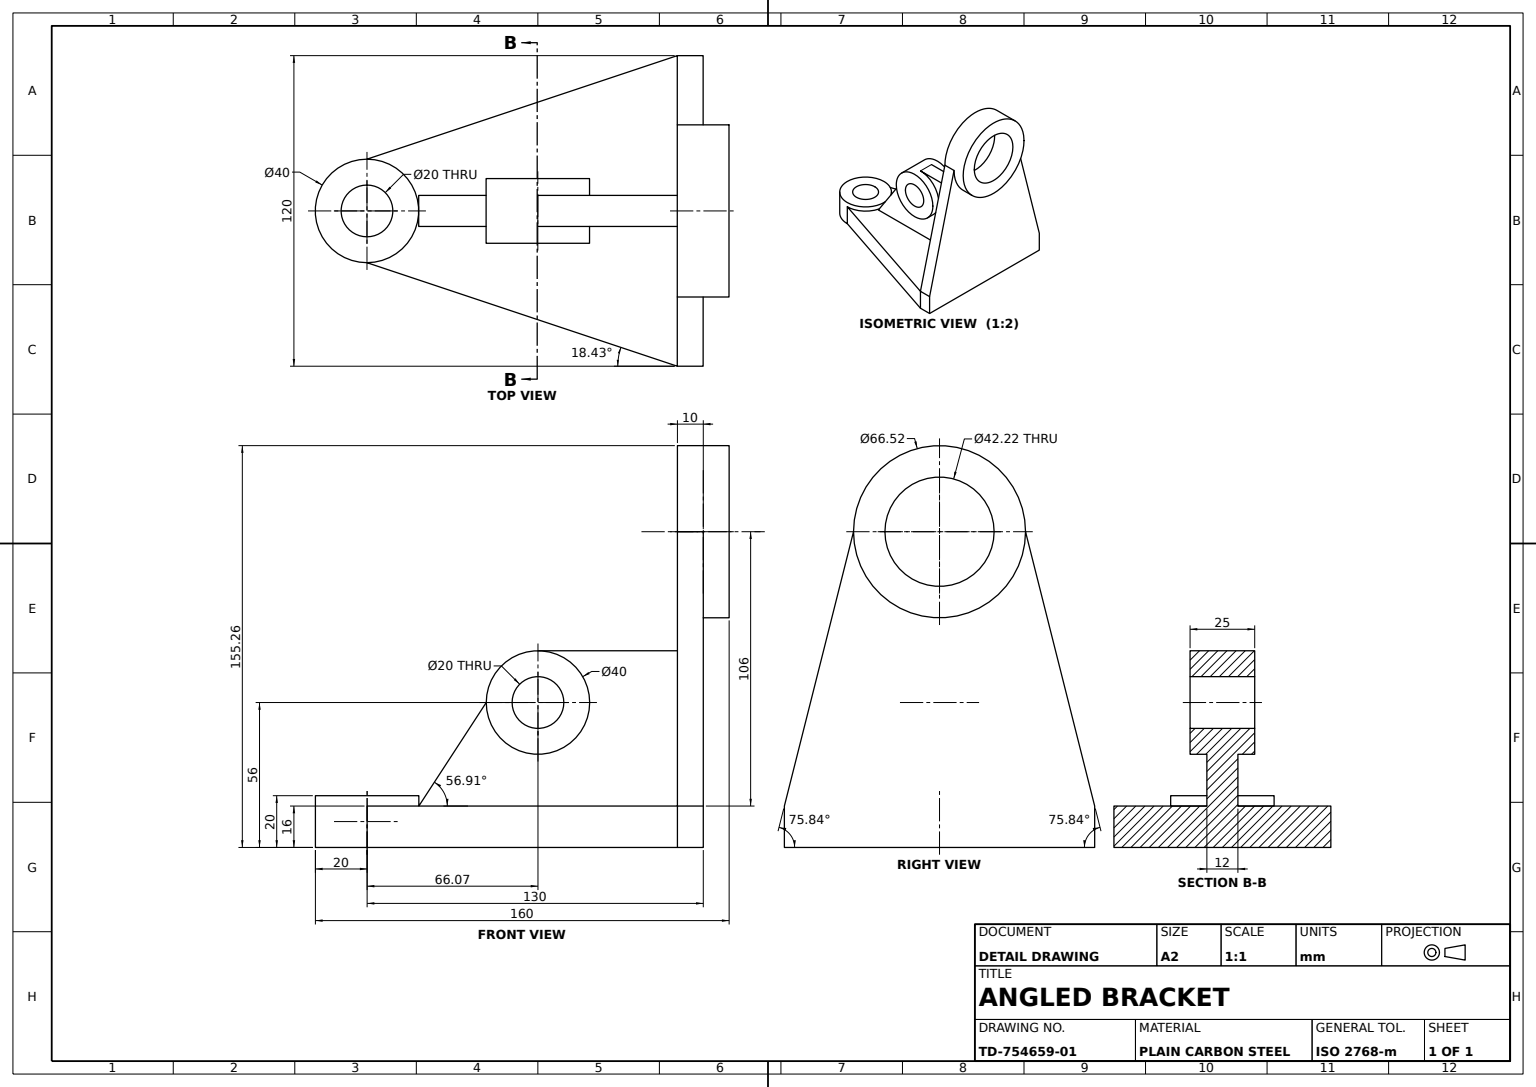
SolidWorks part; units mm, degrees
material "Plain Carbon Steel"
ref_plane "Front Plane" through (0, 0, 0) normal (0, 0, 1) x (1, 0, 0)
ref_plane "Top Plane" through (0, 0, 0) normal (0, 1, 0) x (1, 0, 0)
ref_plane "Right Plane" through (0, 0, 0) normal (1, 0, 0) x (0, 0, -1)
sketch "Base Boss Ring Sketch" plane through (0, 0, 0) normal (0, 1, 0) x (1, 0, 0)
  circle A0 centre (0, 0) radius 20
  circle A1 centre (0, 0) radius 10
  dimension "D1" = 40
  dimension "D2" = 20
extrude "Base Boss Ring Ø40" add sketch "Base Boss Ring Sketch" along normal blind 20
ref_plane "Plane1" through (0, 0, 0) normal (0, 1, 0) x (1, 0, 0)
sketch "Base Plate Sketch" plane through (0, 0, 0) normal (0, 1, 0) x (1, 0, 0)
  line L0 (0, 0) -> (120, 0) construction
  line L2 (120, 60) -> (130, 60)
  line L3 (130, 60) -> (130, -60)
  line L4 (130, -60) -> (120, -60)
  line L6 (0, 20) -> (120, 60)
  line L7 (0, -20) -> (120, -60)
  circle A0 centre (0, 0) radius 20 construction
  arc A1 (0, 20) -> (0, -20) centre (0, 0) cw
  dimension "D1" = 10
  dimension "D2" = 130
extrude "Base Plate" add sketch "Base Plate Sketch" along normal blind 16
ref_plane "Plane2" through (130, 0, 0) normal (1, 0, 0) x (0, 0, -1)
sketch "Upper Boss Ring Sketch" plane through (130, 0, 0) normal (1, 0, 0) x (0, 0, -1)
  line L0 (-60, 16) -> (60, 16) construction
  circle A0 centre (0, 122) radius 21.1123
  circle A1 centre (0, 122) radius 33.2584
  dimension "D1" = 106
  dimension "D2" = 42.2246
  dimension "D3" = 66.5168
extrude "Upper Boss Ring" add sketch "Upper Boss Ring Sketch" along normal mid plane 20 separate body
sketch "Upright Web Sketch" plane through (130, 0, 0) normal (1, 0, 0) x (0, 0, -1)
  line L0 (-60, 16) -> (-33.2584, 122)
  line L1 (60, 16) -> (33.2584, 122)
  line L2 (-60, 16) -> (60, 16)
  line L6 (-60, 0) -> (60, 0)
  line L7 (60, 0) -> (60, 16)
  line L8 (60, 16) -> (-60, 16)
  line L9 (-60, 16) -> (-60, 0)
  line L10 (-60, 0) -> (60, 0)
  circle A0 centre (0, 122) radius 33.2584 construction
  arc A1 (-33.2584, 122) -> (33.2584, 122) centre (0, 122) ccw
  dimension "D1" = 0
extrude "Upright Web" add sketch "Upright Web Sketch" against normal blind 10 contours A1 L0 L2 L1
ref_plane "Plane3" through (0, 0, 0) normal (0, 0, 1) x (1, 0, 0)
sketch "Middle Boss Sketch" plane through (0, 0, 0) normal (0, 0, 1) x (1, 0, 0)
  line L3 (66.07, 76) -> (66.07, 56) construction
  circle A0 centre (66.07, 56) radius 10
  circle A1 centre (66.07, 56) radius 20
  dimension "D1" = 20
  dimension "D2" = 40
  dimension "D3" = 66.07
  dimension "D4" = 56
extrude "Middle Boss" add sketch "Middle Boss Sketch" along normal mid plane 25 separate body
sketch "Gusset Rib Sketch" plane through (0, 0, 0) normal (0, 0, 1) x (1, 0, 0)
  line L0 (66.07, 76) -> (120, 76)
  line L1 (120, 16) -> (120, 122) construction
  line L2 (120, 76) -> (120, 16)
  line L3 (120, 16) -> (20, 16)
  line L4 (20, 16) -> (46.07, 56)
  circle A0 centre (66.07, 56) radius 20 construction
  arc A1 (46.07, 56) -> (66.07, 76) centre (66.07, 56) cw
extrude "Gusset Rib" add sketch "Gusset Rib Sketch" along normal mid plane 12
sketch "Middle Boss Bore Sketch" plane through (0, 0, 6) normal (0, 0, 1) x (1, 0, 0)
  circle A0 centre (66.07, 56) radius 10
  dimension "D1" = 20
extrude "Middle Boss Bore" cut sketch "Middle Boss Bore Sketch" against normal through all
